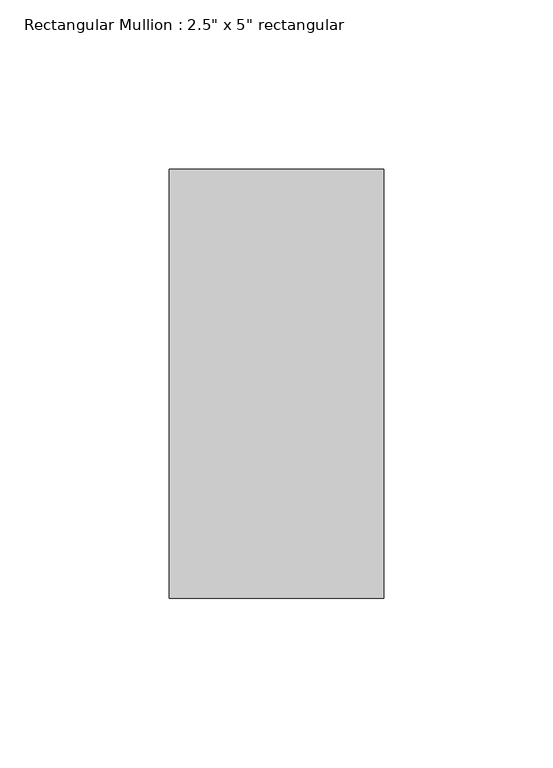
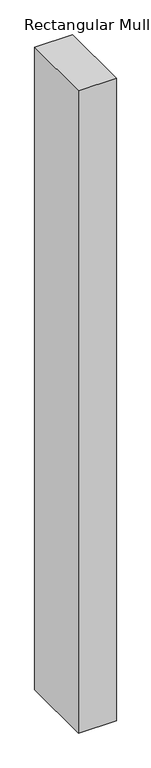
"""IFC4 building model written with IfcOpenShell, lengths in millimetres: member geometry."""

from ifc_helpers import new_model, si_unit, frame, origin, place, context, project, spatial, polyline, outline, extrude, source, transform, mapped, element, save


def member_55de22a4(model_context):
    return source(origin(), model_context, "Body", "SweptSolid", [
        extrude(outline(polyline([(0.0, 63.5), (0.0, -63.5), (-63.5, -63.5), (-63.5, 63.5), (0.0, 63.5)])), frame((0.0, 0.0, -1137.9026335), z_axis=(0.0, 0.0, 1.0), x_axis=(1.0, 0.0, 0.0)), (0.0, 0.0, 1.0), 1137.9026335),
    ])


if __name__ == "__main__":
    model = new_model("IFC4")
    model_context = context("Model", 3, world=origin())
    ifc_project = project(units=[si_unit("LENGTHUNIT", "METRE", prefix="MILLI")], contexts=[model_context])
    site = spatial("IfcSite", under=ifc_project)
    building = spatial("IfcBuilding", under=site)
    placement = place(None, origin())
    member_shape = member_55de22a4(model_context)
    element("IfcMember", 1, ObjectType="Rectangular Mullion : 2.5\" x 5\" rectangular", at=placement, inside=building, context=model_context, shape_type="MappedRepresentation", body=[
        mapped(member_shape, transform((0.0, 0.0, 0.0), x_axis=(1.0, 0.0, 0.0), y_axis=(0.0, 1.0, 0.0), z_axis=(0.0, 0.0, 1.0))),
    ])
    save(model, "model.ifc")

# Revit data of these elements
# Type "Rectangular Mullion : 2.5\" x 5\" rectangular"
#   built-in parameter 1007304 = 0.416667 (stored number, unit not read)
#   built-in parameter 1007301 = 0.104167 (stored number, unit not read)
#   built-in parameter 1007300 = 0.104167 (stored number, unit not read)
# Element 1 (IfcMember, "Rectangular Mullion : 2.5\" x 5\" rectangular")
#   Materials on its faces: "Aluminum"
# Materials
#   "Aluminum": class "Metal", colour RGB 247 247 247, transparency 0, Description = "Aluminum 6061", Cost = 0
